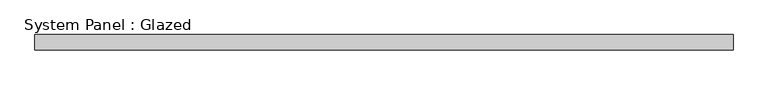
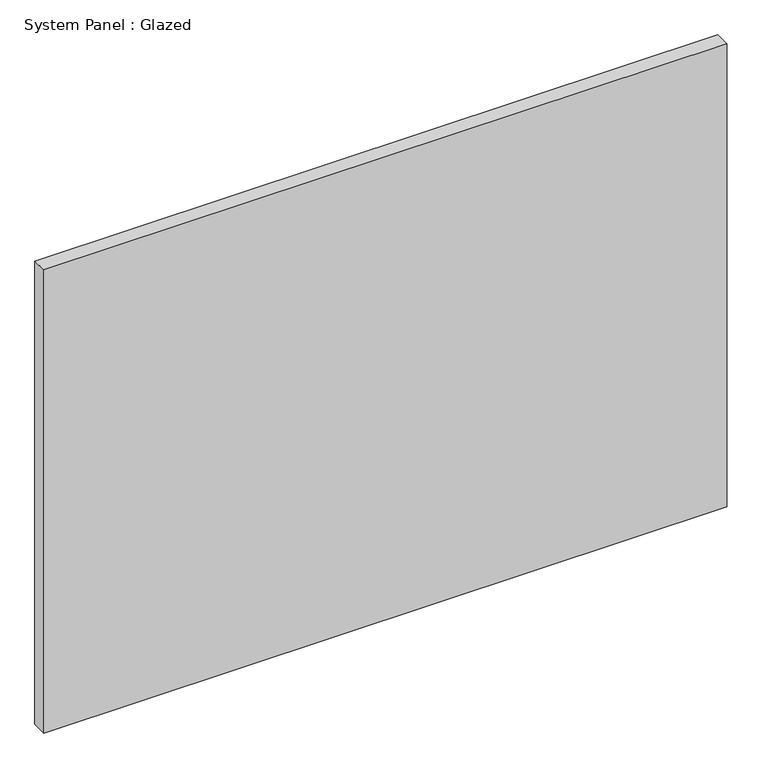
"""IFC4 building model written with IfcOpenShell, lengths in millimetres: plate geometry, System Panel : Glazed."""

from ifc_helpers import new_model, si_unit, origin, origin_with_axes, place, context, project, spatial, polyline, outline, extrude, source, transform, mapped, element, save


def system_panel_glazed_03477ef2(model_context):
    return source(origin(), model_context, "Body", "SweptSolid", [
        extrude(outline(polyline([(571.1875873, 19.05), (-571.1875873, 19.05), (-571.1875873, 44.45), (571.1875873, 44.45), (571.1875873, 19.05)])), origin_with_axes(), (0.0, 0.0, 1.0), 819.15),
    ])


if __name__ == "__main__":
    model = new_model("IFC4")
    model_context = context("Model", 3, world=origin())
    ifc_project = project(units=[si_unit("LENGTHUNIT", "METRE", prefix="MILLI")], contexts=[model_context])
    site = spatial("IfcSite", under=ifc_project)
    building = spatial("IfcBuilding", under=site)
    placement = place(None, origin())
    system_panel_glazed_shape = system_panel_glazed_03477ef2(model_context)
    element("IfcPlate", 1, ObjectType="System Panel : Glazed", at=placement, inside=building, context=model_context, shape_type="MappedRepresentation", body=[
        mapped(system_panel_glazed_shape, transform((0.0, 0.0, 0.0), x_axis=(1.0, 0.0, 0.0), y_axis=(0.0, 1.0, 0.0), z_axis=(0.0, 0.0, 1.0))),
    ])
    save(model, "model.ifc")

# Revit data of these elements
# Type "System Panel : Glazed"
#   Construction Type Id = "GSP4R"
#   Analytic Construction = "1/8 in Pilkington single glazing"
#   Visual Light Transmittance = 0.9
#   Solar Heat Gain Coefficient = 0.86
#   Heat Transfer Coefficient (U) = 1.18115 BTU/(h·ft²·°F)
# Element 1 (IfcPlate, "System Panel : Glazed")
#   Materials on its faces: "Glass"
# Materials
#   "Glass": class "Glass", colour RGB 0 128 192, transparency 0.75, Description = "Soda Lime Glass", Cost = 0
